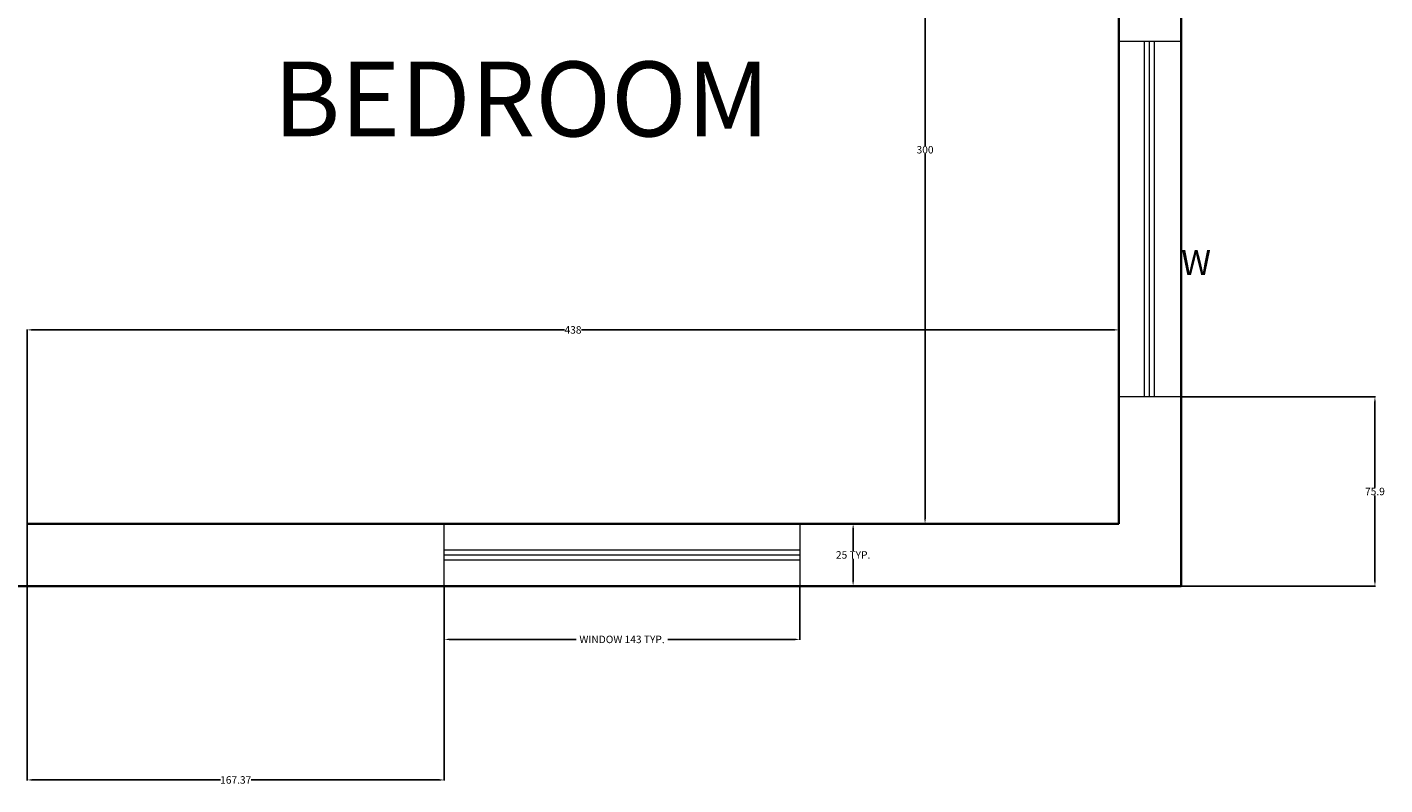
# Model space of a CAD drawing. Units: centimetres. Extents: x -121 to 3851, y -16 to 1180.
# Tile 7 of 16: x 958 to 1503, y -16 to 288. Entities that reach past the tile are written whole.
import ezdxf

# ---------------------------------------------------------------- set-up
doc = ezdxf.new("R2010")
doc.units = ezdxf.units.CM
doc.header["$MEASUREMENT"] = 0
for name, color, linetype, lineweight in [('A-ANNO-DIMS', 2, 'Continuous', 18), ('A-ANNO-IDEN', 3, 'Continuous', 13), ('A-AREA-IDEN', 3, 'Continuous', 18), ('A-GLAZ', 4, 'Continuous', 18), ('A-WALL', 7, 'Continuous', 35)]:
    doc.layers.add(name, color=color, linetype=linetype, lineweight=lineweight)
doc.styles.get("Standard").update_dxf_attribs({"font": 'arial.ttf'})
doc.dimstyles.get("Standard").update_dxf_attribs({"dimtxt": 3, "dimasz": 2, "dimexe": 0.18, "dimexo": 0.0625, "dimgap": 0.09, "dimtad": 0, "dimtih": 1, "dimtoh": 1, "dimdec": 0, "dimzin": 0, "dimdsep": 46, "dimtxsty": 'Standard', "dimcen": 0.09, "dimadec": 0, "dimazin": 0, "dimtfac": 1, "dimtdec": 0, "dimtofl": 0, "dimtmove": 0, "dimatfit": 3, "dimfxl": 1, "dimtolj": 1, "dimtzin": 0, "dimarcsym": 0})

# ---------------------------------------------------------------- blocks, each defined once
blk = doc.blocks.new('WIN-143CM')
for p, q in [((0, 14.5), (142.63, 14.5)), ((0, 12.5), (142.63, 12.5)), ((0, 10.5), (142.63, 10.5))]:
    blk.add_line(p, q)
blk.add_lwpolyline([(0, 25), (142.63, 25), (142.63, 0), (0, 0)], close=True)
blk = doc.blocks.new('*D25')
at = {"layer": 'A-ANNO-DIMS', "color": 0, "lineweight": -2, "transparency": 16777216}
for p, q in [((1125.41, 63.95), (1125.41, 42.44)), ((1268.03, 63.95), (1268.03, 42.44)), ((1127.41, 42.62), (1178.33, 42.62)), ((1266.03, 42.62), (1215.12, 42.62))]:
    blk.add_line(p, q, dxfattribs=at)
at = {"layer": 'A-ANNO-DIMS', "color": 0, "transparency": 16777216}
for points in [[(1127.41, 42.95), (1127.41, 42.29), (1125.41, 42.62)], [(1266.03, 42.95), (1266.03, 42.29), (1268.03, 42.62)]]:
    blk.add_solid(points, dxfattribs=at)
at = {"layer": 'Defpoints', "color": 0, "transparency": 16777216}
for p in [(1125.41, 64.01), (1268.03, 64.01), (1268.03, 42.62)]:
    blk.add_point(p, dxfattribs=at)
at = {"layer": 'A-ANNO-DIMS', "color": 0, "transparency": 16777216, "insert": (1196.72, 42.62), "char_height": 3, "attachment_point": 5}
blk.add_mtext('\\A1;WINDOW 143 TYP.', dxfattribs=at)
blk = doc.blocks.new('*D26')
at = {"layer": 'A-ANNO-DIMS', "color": 0, "lineweight": -2, "transparency": 16777216}
for p, q in [((1268.1, 89.01), (1289.61, 89.01)), ((1289.43, 87.01), (1289.43, 78.14)), ((1289.43, 66.01), (1289.43, 74.89)), ((1268.1, 64.01), (1289.61, 64.01))]:
    blk.add_line(p, q, dxfattribs=at)
at = {"layer": 'A-ANNO-DIMS', "color": 0, "transparency": 16777216}
for points in [[(1289.1, 87.01), (1289.76, 87.01), (1289.43, 89.01)], [(1289.1, 66.01), (1289.76, 66.01), (1289.43, 64.01)]]:
    blk.add_solid(points, dxfattribs=at)
at = {"layer": 'Defpoints', "color": 0, "transparency": 16777216}
for p in [(1268.03, 89.01), (1289.43, 89.01), (1268.03, 64.01)]:
    blk.add_point(p, dxfattribs=at)
at = {"layer": 'A-ANNO-DIMS', "color": 0, "transparency": 16777216, "insert": (1289.43, 76.51), "char_height": 3, "attachment_point": 5}
blk.add_mtext('\\A1;25 TYP.', dxfattribs=at)
blk = doc.blocks.new('*D50')
at = {"layer": 'A-ANNO-DIMS', "color": 0, "lineweight": -2, "transparency": 16777216}
for p, q in [((1420.91, 139.91), (1498.97, 139.91)), ((1498.79, 137.91), (1498.79, 103.58)), ((1498.79, 66.01), (1498.79, 100.34)), ((1421.1, 64.01), (1498.97, 64.01))]:
    blk.add_line(p, q, dxfattribs=at)
at = {"layer": 'A-ANNO-DIMS', "color": 0, "transparency": 16777216}
for points in [[(1498.45, 137.91), (1499.12, 137.91), (1498.79, 139.91)], [(1498.45, 66.01), (1499.12, 66.01), (1498.79, 64.01)]]:
    blk.add_solid(points, dxfattribs=at)
at = {"layer": 'Defpoints', "color": 0, "transparency": 16777216}
for p in [(1420.85, 139.91), (1421.04, 64.01), (1498.79, 64.01)]:
    blk.add_point(p, dxfattribs=at)
at = {"layer": 'A-ANNO-DIMS', "color": 0, "transparency": 16777216, "insert": (1498.79, 101.96), "char_height": 3, "attachment_point": 5}
blk.add_mtext('\\A1;75.9', dxfattribs=at)
blk = doc.blocks.new('*D51')
at = {"layer": 'A-ANNO-DIMS', "color": 0, "lineweight": -2, "transparency": 16777216}
for p, q in [((958.04, 88.95), (958.04, -13.92)), ((1125.41, 63.95), (1125.41, -13.92)), ((960.04, -13.74), (1035.55, -13.74)), ((1123.41, -13.74), (1047.9, -13.74))]:
    blk.add_line(p, q, dxfattribs=at)
at = {"layer": 'A-ANNO-DIMS', "color": 0, "transparency": 16777216}
for points in [[(960.04, -13.4), (960.04, -14.07), (958.04, -13.74)], [(1123.41, -13.4), (1123.41, -14.07), (1125.41, -13.74)]]:
    blk.add_solid(points, dxfattribs=at)
at = {"layer": 'Defpoints', "color": 0, "transparency": 16777216}
for p in [(958.04, 89.01), (1125.41, 64.01), (958.04, -13.74)]:
    blk.add_point(p, dxfattribs=at)
at = {"layer": 'A-ANNO-DIMS', "color": 0, "transparency": 16777216, "insert": (1041.72, -13.74), "char_height": 3, "attachment_point": 5}
blk.add_mtext('\\A1;167.37', dxfattribs=at)
blk = doc.blocks.new('*D60')
at = {"layer": 'A-ANNO-DIMS', "color": 0, "lineweight": -2, "transparency": 16777216}
for p, q in [((958.04, 89.08), (958.04, 166.94)), ((960.04, 166.76), (1173.57, 166.76)), ((1394.04, 166.76), (1180.51, 166.76)), ((1396.04, 89.08), (1396.04, 166.94))]:
    blk.add_line(p, q, dxfattribs=at)
at = {"layer": 'A-ANNO-DIMS', "color": 0, "transparency": 16777216}
for points in [[(960.04, 167.1), (960.04, 166.43), (958.04, 166.76)], [(1394.04, 167.1), (1394.04, 166.43), (1396.04, 166.76)]]:
    blk.add_solid(points, dxfattribs=at)
at = {"layer": 'Defpoints', "color": 0, "transparency": 16777216}
for p in [(1396.04, 166.76), (958.04, 89.01), (1396.04, 89.01)]:
    blk.add_point(p, dxfattribs=at)
at = {"layer": 'A-ANNO-DIMS', "color": 0, "transparency": 16777216, "insert": (1177.04, 166.76), "char_height": 3, "attachment_point": 5}
blk.add_mtext('\\A1;438', dxfattribs=at)
blk = doc.blocks.new('*D61')
at = {"layer": 'A-ANNO-DIMS', "color": 0, "lineweight": -2, "transparency": 16777216}
for p, q in [((1395.98, 389.01), (1318.11, 389.01)), ((1318.29, 387.01), (1318.29, 240.64)), ((1318.29, 91.01), (1318.29, 237.39)), ((1395.98, 89.01), (1318.11, 89.01))]:
    blk.add_line(p, q, dxfattribs=at)
at = {"layer": 'A-ANNO-DIMS', "color": 0, "transparency": 16777216}
for points in [[(1317.95, 387.01), (1318.62, 387.01), (1318.29, 389.01)], [(1317.95, 91.01), (1318.62, 91.01), (1318.29, 89.01)]]:
    blk.add_solid(points, dxfattribs=at)
at = {"layer": 'Defpoints', "color": 0, "transparency": 16777216}
for p in [(1318.29, 389.01), (1396.04, 389.01), (1396.04, 89.01)]:
    blk.add_point(p, dxfattribs=at)
at = {"layer": 'A-ANNO-DIMS', "color": 0, "transparency": 16777216, "insert": (1318.29, 239.01), "char_height": 3, "attachment_point": 5}
blk.add_mtext('\\A1;300', dxfattribs=at)

msp = doc.modelspace()

# ---------------------------------------------------------------- linework, layer by layer
at = {"layer": 'A-WALL'}
for p, q in [((1421.0382, 880.0141), (1421.0382, 64.0141)), ((1396.0382, 389.0141), (1396.0382, 89.0141)), ((1396.0382, 89.0141), (958.0382, 89.0141)), ((1421.0382, 64.0141), (65.0382, 64.0141))]:
    msp.add_line(p, q, dxfattribs=at)

# ---------------------------------------------------------------- block references
at = {"layer": 'A-GLAZ', "rotation": 90.0000000000001}
msp.add_blockref('WIN-143CM', (1420.8472, 139.9088), dxfattribs=at)
at = {"layer": 'A-GLAZ'}
msp.add_blockref('WIN-143CM', (1125.4064, 64.014), dxfattribs=at)

# ---------------------------------------------------------------- texts
at = {"layer": 'A-ANNO-IDEN', "insert": (1421.0382, 198.7842), "char_height": 10, "attachment_point": 1}
msp.add_mtext_dynamic_manual_height_columns('W', width=55.718495, gutter_width=1, heights=[0], dxfattribs=at)
at = {"layer": 'A-AREA-IDEN', "insert": (1056.8028, 274.3772), "char_height": 30, "attachment_point": 1}
msp.add_mtext_dynamic_manual_height_columns('BEDROOM', width=248.976965, gutter_width=1, heights=[0], dxfattribs=at)

# ---------------------------------------------------------------- dimensions: what is measured, and where the dimension line sits
at = {"layer": 'A-ANNO-DIMS'}
for base, p1, p2, override, picture, middle in [((1318.2882, 389.0141), (1396.0382, 89.0141), (1396.0382, 389.0141), {"dimdec": 0, "dimlfac": 1, "dimrnd": 0, "dimzin": 0, "dimdsep": 46, "dimlunit": 2}, '*D61', (1318.2882, 239.0141)), ((1498.7882, 64.0141), (1420.8471, 139.9089), (1421.0382, 64.0141), {"dimdec": 1, "dimlfac": 1, "dimrnd": 0, "dimzin": 0, "dimdsep": 46, "dimlunit": 2}, '*D50', (1498.7882, 101.9615))]:
    dim = msp.add_linear_dim(base=base, p1=p1, p2=p2, angle=90, dimstyle='Standard', override=override, dxfattribs=at)
    dim.commit()
    dim.dimension.update_dxf_attribs({"geometry": picture, "text_midpoint": middle})
for base, p1, p2, override, picture, middle in [((1396.0382, 166.7641), (958.0382, 89.0141), (1396.0382, 89.0141), {"dimdec": 0, "dimlfac": 1, "dimrnd": 0, "dimzin": 0, "dimdsep": 46, "dimlunit": 2}, '*D60', (1177.0382, 166.7641)), ((958.0382, -13.7359), (1125.4065, 64.0141), (958.0382, 89.0141), {"dimdec": 2, "dimlfac": 1, "dimrnd": 0, "dimzin": 0, "dimdsep": 46, "dimlunit": 2}, '*D51', (1041.7223, -13.7359))]:
    dim = msp.add_linear_dim(base=base, p1=p1, p2=p2, dimstyle='Standard', override=override, dxfattribs=at)
    dim.commit()
    dim.dimension.update_dxf_attribs({"geometry": picture, "text_midpoint": middle})
dim = msp.add_linear_dim(base=(1289.4289, 89.0141), p1=(1268.0346, 64.0141), p2=(1268.0346, 89.0141), angle=90, text='<> TYP.', dimstyle='Standard', override={"dimdec": 0, "dimlfac": 1, "dimrnd": 0, "dimzin": 0, "dimdsep": 46, "dimlunit": 2}, dxfattribs=at)
dim.commit()
dim.dimension.update_dxf_attribs({"geometry": '*D26', "text_midpoint": (1289.4289, 76.5141)})
dim = msp.add_linear_dim(base=(1268.0346, 42.6199), p1=(1125.4065, 64.0141), p2=(1268.0346, 64.0141), text='WINDOW <> TYP.', dimstyle='Standard', override={"dimdec": 0, "dimlfac": 1, "dimrnd": 0, "dimzin": 0, "dimdsep": 46, "dimlunit": 2}, dxfattribs=at)
dim.commit()
dim.dimension.update_dxf_attribs({"geometry": '*D25', "text_midpoint": (1196.7205, 42.6199)})

doc.saveas('drawing.dxf')
